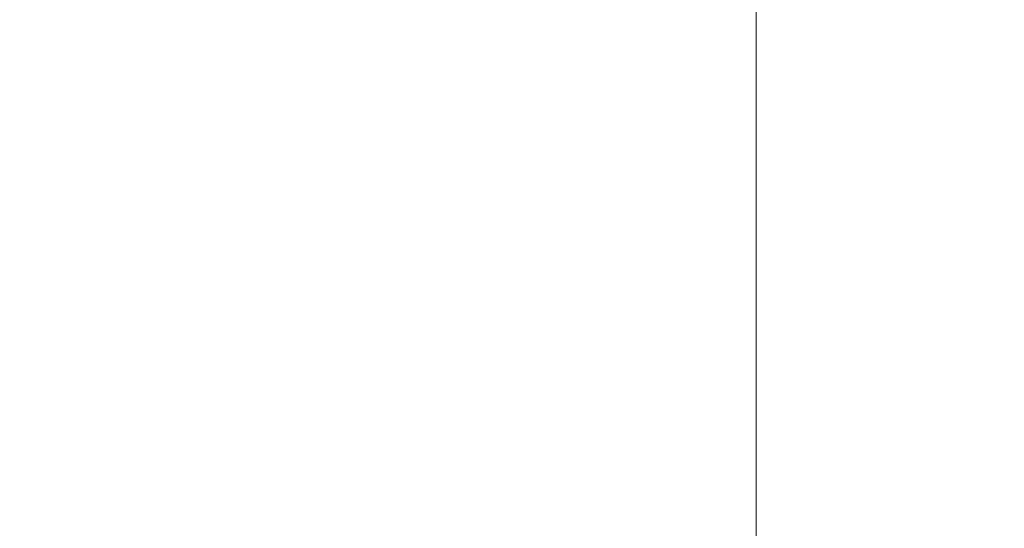
# Model space of a CAD drawing. Units: inches. Extents: x -466983 to 1020, y 324 to 318697.
# Tile 53 of 97: x 631.804 to 637.858, y 936.436 to 939.565. Entities that reach past the tile are written whole.
import ezdxf

# ---------------------------------------------------------------- set-up
doc = ezdxf.new("R2010")
doc.units = ezdxf.units.IN
doc.header["$MEASUREMENT"] = 0
doc.layers.add('A-FLOR-PATT', color=252, linetype='Continuous', lineweight=13)
doc.layers.add('A-FURN', color=8, linetype='Continuous', lineweight=18)

# ---------------------------------------------------------------- blocks, each defined once
blk = doc.blocks.new('L Shaped Sofa')
at = {"ltscale": 2}
blk.add_line((2432.347, 748.121), (2432.347, 765.179), dxfattribs=at)

msp = doc.modelspace()

# ---------------------------------------------------------------- hatches: boundary and pattern name
at = {"layer": 'A-FLOR-PATT', "transparency": 33554572}
h = msp.add_hatch(dxfattribs=at)
h.set_pattern_fill('ANSI37', color=256, scale=30)
h.set_pattern_definition([(45, (-1212.4137, -290.035), (-2.6516504, 2.6516504), []), (135, (-1212.4137, -290.035), (-2.6516504, -2.6516504), [])])
h.paths.add_polyline_path([(901.8057, 1075.9377), (900.6144, 1075.9377), (900.6144, 1065.3856), (899.391, 1065.3856), (898.0911, 1065.3856), (892.8356, 1058.7098, -0.258377), (892.1875, 1058.3509), (879.9848, 1058.3509, -0.20177), (879.4382, 1058.5808), (874.0812, 1065.3856), (872.7813, 1065.3856), (871.5579, 1065.3856), (871.5579, 1075.9377), (813.8057, 1075.9377), (813.8057, 1044.7922), (832.3947, 1044.7922, -0.394795), (848.6602, 1028.5356), (848.6602, 1009.9377), (901.8057, 1009.9377), (901.8057, 1015.9377), (901.3057, 1015.9377), (871.3057, 1015.9377), (871.3057, 1017.2502), (871.3344, 1017.2502, -0.401453), (901.3057, 1045.9377), (901.8057, 1045.9377)])
edge = h.paths.add_edge_path(flags=16)
edge.add_line((847.7731, 1068.9486), (847.7731, 1073.7088))
edge.add_arc((849.2269, 1073.7088), 1.4538, 90, 180, ccw=False)
edge.add_line((849.2269, 1075.1627), (864.4921, 1075.1627))
edge.add_arc((864.4921, 1073.7088), 1.4538, 0, 90, ccw=False)
edge.add_line((865.9459, 1073.7088), (865.9459, 1069.0035))
edge.add_arc((832.6447, 1068.9761), 33.3012, -20.61234, 0.04725, ccw=False)
edge.add_ellipse((856.8595, 1058.48), major_axis=(0, 10.2131), ratio=0.6859192, start_angle=100.00884, end_angle=259.99116, ccw=False)
edge.add_arc((881.0742, 1068.9761), 33.3012, 180.04725, 200.61234, ccw=False)
h.paths.add_polyline_path([(853.1456, 1066.4815), (853.1456, 1066.4534), (853.1463, 1066.4534, 0.433107), (852.9166, 1066.6849), (852.9166, 1066.4534), (853.1456, 1066.4534), (853.1456, 1066.4815), (853.088, 1066.6122, 0.697939), (852.6995, 1066.4534), (852.7003, 1066.4534), (852.7003, 1066.4815), (852.9166, 1067.0012), (852.9166, 1066.6849, -0.396254)], flags=0)
h.paths.add_polyline_path([(861.0187, 1066.4815), (861.0187, 1066.4534), (861.0194, 1066.4534, 0.416404), (860.8024, 1066.6849), (860.8024, 1066.4534), (861.0187, 1066.4534), (861.0187, 1066.4815), (860.9672, 1066.6053, 0.713344), (860.5726, 1066.4534), (860.5734, 1066.4534), (860.5734, 1066.4815), (860.8024, 1067.0012), (860.8024, 1066.6849, -0.379973)], flags=0)
edge = h.paths.add_edge_path(flags=0)
edge.add_spline(control_points=[(861.1298, 1065.7855), (861.4661, 1065.2478), (861.6134, 1065.0161), (861.9833, 1064.3736), (862.1924, 1063.9443), (862.5614, 1063.0391), (862.7212, 1062.5633), (862.9865, 1061.5781), (863.092, 1061.0689), (863.2452, 1060.031), (863.293, 1059.5025), (863.3295, 1058.4409), (863.3181, 1057.9078), (863.2366, 1056.8518), (863.1664, 1056.3289), (862.9695, 1055.308), (862.8427, 1054.8099), (862.5365, 1053.8522), (862.3571, 1053.3927), (861.9514, 1052.5249), (861.7251, 1052.1166), (861.233, 1051.3622), (860.9672, 1051.0162), (860.4048, 1050.3949), (860.1082, 1050.1197), (859.4937, 1049.6461), (859.1758, 1049.4476), (858.5276, 1049.1299), (858.1973, 1049.0107), (857.5315, 1048.8518), (857.1959, 1048.8121), (856.5249, 1048.812), (856.1894, 1048.8515), (855.5236, 1049.0101), (855.1933, 1049.1291), (854.545, 1049.4465), (854.2271, 1049.6449), (853.6124, 1050.1183), (853.3158, 1050.3933), (852.7533, 1051.0143), (852.4874, 1051.3602), (851.9952, 1052.1144), (851.7688, 1052.5225), (851.3629, 1053.3902), (851.1834, 1053.8496), (850.877, 1054.8071), (850.7501, 1055.3051), (850.553, 1056.326), (850.4827, 1056.8488), (850.401, 1057.9048), (850.3895, 1058.4379), (850.4257, 1059.4995), (850.4734, 1060.0281), (850.6265, 1061.066), (850.7318, 1061.5753), (850.9969, 1062.5605), (851.1567, 1063.0365), (851.5254, 1063.9418), (851.7345, 1064.3712), (852.1056, 1065.0164), (852.2544, 1065.2503), (852.6082, 1065.7335)], knot_values=[3.915332, 3.915332, 3.915332, 3.915332, 4.013468, 4.013468, 4.175532, 4.175532, 4.337596, 4.337596, 4.49966, 4.49966, 4.661724, 4.661724, 4.823788, 4.823788, 4.985852, 4.985852, 5.147916, 5.147916, 5.30998, 5.30998, 5.472044, 5.472044, 5.634109, 5.634109, 5.796173, 5.796173, 5.958237, 5.958237, 6.120301, 6.120301, 6.282365, 6.282365, 6.444429, 6.444429, 6.606493, 6.606493, 6.768557, 6.768557, 6.930621, 6.930621, 7.092685, 7.092685, 7.254749, 7.254749, 7.416813, 7.416813, 7.578878, 7.578878, 7.740942, 7.740942, 7.903006, 7.903006, 8.06507, 8.06507, 8.227134, 8.227134, 8.389198, 8.389198, 8.551262, 8.551262, 8.65037, 8.65037, 8.65037, 8.65037], degree=3, periodic=0)
edge.add_line((852.6421, 1065.7855), (861.1298, 1065.7855))
edge = h.paths.add_edge_path(flags=0)
edge.add_ellipse((856.8496, 1057.7432), major_axis=(0, 7.7921), ratio=0.687861, start_angle=0, end_angle=360)
h.paths.add_polyline_path([(848.8634, 1069.3891), (848.8634, 1073.9605, -0.414214), (849.9538, 1075.0508), (863.7652, 1075.0508, -0.414214), (864.8555, 1073.9605), (864.8555, 1069.3891, -0.388936), (864.5237, 1069.027, -0.043561), (849.1953, 1069.027, -0.388936)], flags=0)
h.paths.add_polyline_path([(853.1006, 1068.1122, -1), (852.6775, 1068.1122, -1)], flags=0)
edge = h.paths.add_edge_path(flags=0)
edge.add_ellipse((856.8595, 1057.3378), major_axis=(0, 2.207), ratio=0.657164, start_angle=0, end_angle=360)
h.paths.add_polyline_path([(861.0415, 1068.1122, -1), (860.6184, 1068.1122, -1)], flags=0)
edge = h.paths.add_edge_path()
edge.add_line((573.9537, 1057.3412), (573.9537, 1075.9377))
edge.add_line((573.9537, 1075.9377), (558.7308, 1075.9377))
edge.add_line((558.7308, 1075.9377), (558.7308, 1065.3856))
edge.add_line((558.7308, 1065.3856), (557.5074, 1065.3856))
edge.add_line((557.5074, 1065.3856), (556.2075, 1065.3856))
edge.add_line((556.2075, 1065.3856), (550.952, 1058.7098))
edge.add_arc((550.3039, 1059.1155), 0.7646, 270, 327.94832, ccw=False)
edge.add_line((550.3039, 1058.3509), (538.1012, 1058.3509))
edge.add_arc((538.1012, 1059.1155), 0.7646, 224.3704, 270, ccw=False)
edge.add_line((537.5546, 1058.5808), (532.1976, 1065.3856))
edge.add_line((532.1976, 1065.3856), (530.8977, 1065.3856))
edge.add_line((530.8977, 1065.3856), (529.6743, 1065.3856))
edge.add_line((529.6743, 1065.3856), (529.6743, 1075.9377))
edge.add_line((529.6743, 1075.9377), (520.8057, 1075.9377))
edge.add_line((520.8057, 1075.9377), (520.8057, 1045.9377))
edge.add_line((520.8057, 1045.9377), (521.3057, 1045.9377))
edge.add_arc((521.3057, 1015.9377), 30, 2.50749, 90, ccw=False)
edge.add_line((551.277, 1017.2502), (551.3057, 1017.2502))
edge.add_line((551.3057, 1017.2502), (551.3057, 1015.9377))
edge.add_line((551.3057, 1015.9377), (520.8057, 1015.9377))
edge.add_line((520.8057, 1015.9377), (520.8057, 1009.9377))
edge.add_line((520.8057, 1009.9377), (559.1913, 1010.4022))
edge.add_arc((559.1913, 1011.856), 1.4538, 180, 270, ccw=False)
edge.add_line((557.7375, 1011.856), (557.7375, 1016.5613))
edge.add_arc((591.0386, 1016.5888), 33.3012, 159.38766, 180.04725, ccw=False)
edge.add_ellipse((566.8239, 1027.0848), major_axis=(0, 10.2131), ratio=0.6859192, start_angle=280.00884, end_angle=439.99116, ccw=False)
edge.add_arc((542.6091, 1016.5888), 33.3012, 0.04725, 20.61234, ccw=False)
edge.add_line((575.9103, 1016.6162), (575.9103, 1011.856))
edge.add_arc((574.4565, 1011.856), 1.4538, -90, 0, ccw=False)
edge.add_line((574.4565, 1010.4022), (608.8057, 1009.9377))
edge.add_line((608.8057, 1009.9377), (608.8057, 1041.0857))
edge.add_line((608.8057, 1041.0857), (590.2179, 1041.0857))
edge.add_arc((590.775, 1057.9074), 16.8309, 181.92775, 268.10321, ccw=False)
edge = h.paths.add_edge_path()
edge.add_ellipse((494.2443, 583.6204), major_axis=(0, 10.2131), ratio=0.6859192, start_angle=280.00884, end_angle=439.99116, ccw=False)
edge.add_arc((470.0296, 573.1243), 33.3012, 0.04725, 20.61234, ccw=False)
edge.add_line((503.3307, 573.1518), (503.3307, 568.3916))
edge.add_arc((501.8769, 568.3916), 1.4538, -90, 0, ccw=False)
edge.add_line((501.8769, 566.9377), (539.8057, 566.9377))
edge.add_line((539.8057, 566.9377), (539.8057, 572.9377))
edge.add_line((539.8057, 572.9377), (539.3057, 572.9377))
edge.add_line((539.3057, 572.9377), (509.3057, 572.9377))
edge.add_line((509.3057, 572.9377), (509.3057, 574.2502))
edge.add_line((509.3057, 574.2502), (509.3344, 574.2502))
edge.add_arc((539.3057, 572.9377), 30, 90, 177.49251, ccw=False)
edge.add_line((539.3057, 602.9377), (539.8057, 602.9377))
edge.add_line((539.8057, 602.9377), (539.8057, 626.9377))
edge.add_line((539.8057, 626.9377), (531.7718, 626.9377))
edge.add_line((531.7718, 626.9377), (531.7718, 616.3856))
edge.add_line((531.7718, 616.3856), (530.5484, 616.3856))
edge.add_line((530.5484, 616.3856), (529.2485, 616.3856))
edge.add_line((529.2485, 616.3856), (523.7105, 609.3509))
edge.add_line((523.7105, 609.3509), (510.7766, 609.3509))
edge.add_line((510.7766, 609.3509), (505.2386, 616.3856))
edge.add_line((505.2386, 616.3856), (503.9387, 616.3856))
edge.add_line((503.9387, 616.3856), (502.7153, 616.3856))
edge.add_line((502.7153, 616.3856), (502.7153, 626.9377))
edge.add_line((502.7153, 626.9377), (481.6983, 626.9377))
edge.add_line((481.6983, 626.9377), (481.6983, 610.995))
edge.add_arc((467.2703, 611.4728), 14.4359, 271.92775, 358.10321, ccw=False)
edge.add_line((467.7559, 597.0451), (451.8057, 597.0451))
edge.add_line((451.8057, 597.0451), (451.8057, 584.4035))
edge.add_line((451.8057, 584.4035), (451.8057, 566.9377))
edge.add_line((451.8057, 566.9377), (486.6117, 566.9377))
edge.add_arc((486.6117, 568.3916), 1.4538, 180, 270, ccw=False)
edge.add_line((485.1579, 568.3916), (485.1579, 573.0969))
edge.add_arc((518.4591, 573.1243), 33.3012, 159.38766, 180.04725, ccw=False)
h.paths.add_polyline_path([(836.2609, 1020.7328), (879.8898, 1020.7328), (879.8898, 1039.3902), (836.2609, 1039.3902)], flags=25)
h.paths.add_polyline_path([(549.9851, 1036.7492), (593.614, 1036.7492), (593.614, 1055.4065), (549.9851, 1055.4065)], flags=24)
h.paths.add_polyline_path([(475.123, 595.5959), (518.752, 595.5959), (518.752, 614.2532), (475.123, 614.2532)], flags=24)
h = msp.add_hatch(dxfattribs=at)
h.set_pattern_fill('ANSI37', color=256, scale=20)
h.set_pattern_definition([(45, (-1212.4137, -290.035), (-1.767767, 1.767767), []), (135, (-1212.4137, -290.035), (-1.767767, -1.767767), [])])
h.paths.add_polyline_path([(809.8057, 870.9377), (809.8057, 888.1519), (806.9985, 888.1519), (802.6624, 888.1519), (789.3832, 888.1519), (786.2846, 888.1519, -0.414214), (785.4991, 888.9374), (785.4991, 900.1959), (785.4991, 908.4696, -0.414214), (786.8082, 909.7787, -0.414214), (785.4991, 911.0878), (785.4991, 929.1015, -0.414214), (786.8082, 930.4106, -0.414214), (785.4991, 931.7197), (785.4991, 931.9039, -0.414214), (784.19, 930.5948), (766.7223, 930.5948, -0.412359), (765.4132, 931.8956, -0.413741), (764.1145, 930.5782), (744.5781, 930.422, -0.416556), (743.7864, 931.2075), (743.7864, 933.5153), (742.2154, 933.5153), (742.2154, 952.024, -0.001344), (743.7864, 952.1998), (743.7864, 953.9377), (678.5915, 953.9377), (678.5915, 951.1305), (678.5915, 946.7945), (678.5915, 933.5153), (678.5915, 930.4166, -0.414214), (677.806, 929.6312), (666.5475, 929.6312), (658.2738, 929.6312, -0.414214), (656.9647, 930.9403, -0.414214), (655.6556, 929.6312), (637.6419, 929.6312, -0.414214), (636.3328, 930.9403, -0.414214), (635.0237, 929.6312), (634.8395, 929.6312, -0.414214), (636.1486, 928.322), (636.1486, 910.8544, -0.412359), (634.8478, 909.5452, -0.413741), (636.1653, 908.2466), (636.3214, 888.7102, -0.416556), (635.5359, 887.9184), (633.2281, 887.9184), (633.2281, 886.3475), (614.7194, 886.3475, -0.001344), (614.5436, 887.9184), (612.8057, 887.9184), (612.8057, 834.9377), (612.8057, 752.9377), (612.8057, 748.9377), (612.8057, 697.9377), (654.8057, 697.9377), (654.8057, 701.9377), (715.8057, 701.9377), (715.8057, 737.4353), (774.2918, 737.4353), (774.2918, 795.9377), (809.8057, 795.9377)])
h.paths.add_polyline_path([(679.2761, 849.5757, 0.102523), (682.1475, 849.2608, -0.080461), (694.5428, 849.7725, -0.283899), (694.4822, 849.0082, 0.136605), (694.4068, 848.8103, -0.030441), (694.5428, 846.8929), (694.5428, 842.6198), (694.5428, 838.3466, -0.028219), (694.4246, 836.5684), (694.425, 836.5684, 0.196187), (694.4456, 836.2708, -0.302897), (694.5428, 835.467, -0.080461), (682.1475, 835.9787, 0.102523), (679.2761, 835.6638, -0.58611), (678.6457, 836.0169), (678.6457, 849.2227, -0.58611)], flags=16)
h.paths.add_polyline_path([(679.5173, 848.6515, 0.699597), (679.476, 848.6342, 1.20716), (679.1935, 848.7422, 0.010621)], flags=0)
h.paths.add_polyline_path([(679.4923, 836.5608, -0.013798), (679.9178, 836.6594, -0.071703), (682.8533, 837.1434, -0.165743), (682.1665, 839.1006), (682.1665, 842.6094), (682.1665, 846.0603, -0.240616), (683.4733, 848.6767, -0.068263), (693.9295, 849.0082), (693.7875, 848.7083), (693.7875, 849.0228, 0.067332), (683.4733, 848.6767, 0.240616), (682.1665, 846.0603), (682.1665, 842.6094), (682.1665, 839.1006, 0.23459), (683.461, 836.5513, 0.068093), (693.7875, 836.1955), (693.7875, 836.5104), (693.9296, 836.2102, -0.077215), (682.2421, 836.7815, 0.086627), (679.5283, 836.5701, -0.628402), (679.5029, 836.5735), (679.5029, 836.6071, 0.910458)], flags=0)
h.paths.add_polyline_path([(679.476, 848.6364), (679.2069, 848.647), (679.2069, 836.5718, 0.913566), (679.3645, 836.5861), (679.476, 836.5824)], flags=0)
h.paths.add_polyline_path([(679.2761, 829.8604, 0.102523), (682.1475, 829.5455, -0.080461), (694.5428, 830.0572, -0.283899), (694.4822, 829.2929, 0.136605), (694.4068, 829.095, -0.030441), (694.5428, 827.1776), (694.5428, 822.9045), (694.5428, 818.6314, -0.028219), (694.4246, 816.8531), (694.425, 816.8532, 0.196187), (694.4456, 816.5555, -0.302897), (694.5428, 815.7517, -0.080461), (682.1475, 816.2635, 0.102523), (679.2761, 815.9485, -0.58611), (678.6457, 816.3016), (678.6457, 829.5074, -0.58611)], flags=16)
h.paths.add_polyline_path([(679.5173, 828.9362, 0.699597), (679.476, 828.9189, 1.20716), (679.1935, 829.0269, 0.010621)], flags=0)
h.paths.add_polyline_path([(679.4923, 816.8456, -0.013798), (679.9178, 816.9441, -0.071703), (682.8533, 817.4281, -0.165743), (682.1665, 819.3853), (682.1665, 822.8941), (682.1665, 826.345, -0.240616), (683.4733, 828.9614, -0.068263), (693.9295, 829.2929), (693.7875, 828.9931), (693.7875, 829.3076, 0.067332), (683.4733, 828.9614, 0.240616), (682.1665, 826.345), (682.1665, 822.8941), (682.1665, 819.3853, 0.23459), (683.461, 816.836, 0.068093), (693.7875, 816.4802), (693.7875, 816.7952), (693.9296, 816.4949, -0.077215), (682.2421, 817.0662, 0.086627), (679.5283, 816.8549, -0.628402), (679.5029, 816.8582), (679.5029, 816.8918, 0.910458)], flags=0)
h.paths.add_polyline_path([(679.476, 828.9211), (679.2069, 828.9317), (679.2069, 816.8565, 0.913566), (679.3645, 816.8708), (679.476, 816.8671)], flags=0)
h.paths.add_polyline_path([(679.2761, 810.1451, 0.102523), (682.1475, 809.8302, -0.080461), (694.5428, 810.342, -0.3023), (694.4466, 809.5394, 0.10023), (694.4058, 809.3878, -0.03057), (694.5428, 807.4623), (694.5428, 803.1892), (694.5428, 798.9161, -0.03057), (694.4058, 796.9906, 0.10023), (694.4466, 796.839, -0.3023), (694.5428, 796.0365, -0.080461), (682.1475, 796.5482, 0.102523), (679.2761, 796.2333, -0.58611), (678.6457, 796.5863), (678.6457, 809.7921, -0.58611)], flags=16)
h.paths.add_polyline_path([(679.5173, 809.2417, 0.699597), (679.476, 809.2244, 1.20716), (679.1935, 809.3324, 0.010621)], flags=0)
h.paths.add_polyline_path([(679.4923, 797.151, -0.013798), (679.9178, 797.2496, -0.071703), (682.8533, 797.7336, -0.165743), (682.1665, 799.6908), (682.1665, 803.1996), (682.1665, 806.6505, -0.239349), (683.461, 809.2577, -0.072465), (694.4468, 809.5405, 0.197932), (694.425, 809.2405), (693.7875, 809.2985), (693.7875, 809.6135, 0.068093), (683.461, 809.2577, 0.239349), (682.1665, 806.6505), (682.1665, 803.1996), (682.1665, 799.6908, 0.235854), (683.4733, 797.1323, 0.067332), (693.7875, 796.7861), (693.7875, 797.1006), (694.425, 797.1586, 0.197932), (694.4468, 796.8586, -0.080419), (682.1557, 797.3795, 0.083867), (679.5283, 797.1603, -0.628402), (679.5029, 797.1637), (679.5029, 797.1973, 0.910458)], flags=0)
h.paths.add_polyline_path([(679.2069, 809.2372), (679.2069, 797.162, 0.913566), (679.3645, 797.1763), (679.476, 797.1726), (679.476, 809.2266)], flags=0)
h.paths.add_polyline_path([(695.3643, 853.2989), (728.2231, 853.2989), (728.2231, 771.1519), (695.3643, 771.1519)], flags=16)
h.paths.add_polyline_path([(696.0215, 852.6417), (727.5659, 852.6417), (727.5659, 771.809), (696.0215, 771.809)], flags=0)
h.paths.add_polyline_path([(679.2761, 788.7869, 0.102523), (682.1475, 788.472, -0.080461), (694.5428, 788.9837, -0.3023), (694.4466, 788.1812, 0.10023), (694.4058, 788.0296, -0.03057), (694.5428, 786.1041), (694.5428, 781.831), (694.5428, 777.5578, -0.03057), (694.4058, 775.6323, 0.10023), (694.4466, 775.4808, -0.3023), (694.5428, 774.6782, -0.080461), (682.1475, 775.19, 0.102523), (679.2761, 774.875, -0.58611), (678.6457, 775.2281), (678.6457, 788.4339, -0.58611)], flags=16)
h.paths.add_polyline_path([(679.5173, 787.8834, 0.699597), (679.476, 787.8662, 1.20716), (679.1935, 787.9742, 0.010621)], flags=0)
h.paths.add_polyline_path([(679.4923, 775.7928, -0.013798), (679.9178, 775.8914, -0.071703), (682.8533, 776.3753, -0.165743), (682.1665, 778.3325), (682.1665, 781.8414), (682.1665, 785.2922, -0.239349), (683.461, 787.8995, -0.072465), (694.4468, 788.1823, 0.197932), (694.425, 787.8823), (693.7875, 787.9403), (693.7875, 788.2553, 0.068093), (683.461, 787.8995, 0.239349), (682.1665, 785.2922), (682.1665, 781.8414), (682.1665, 778.3325, 0.235854), (683.4733, 775.7741, 0.067332), (693.7875, 775.4279), (693.7875, 775.7424), (694.425, 775.8004, 0.197932), (694.4468, 775.5004, -0.080419), (682.1557, 776.0212, 0.083867), (679.5283, 775.8021, -0.628402), (679.5029, 775.8054), (679.5029, 775.8391, 0.910458)], flags=0)
h.paths.add_polyline_path([(679.2069, 787.8789), (679.2069, 775.8038, 0.913566), (679.3645, 775.818), (679.476, 775.8144), (679.476, 787.8684)], flags=0)
h.paths.add_polyline_path([(704.641, 854.1204, -0.080461), (705.1527, 866.5157, 0.102523), (704.8378, 869.3871, -0.58611), (705.1908, 870.0174), (718.3966, 870.0174, -0.58611), (718.7496, 869.3871, 0.102523), (718.4347, 866.5157, -0.080461), (718.9465, 854.1204, -0.3023), (718.1439, 854.2166, 0.10023), (717.9924, 854.2574, -0.03057), (716.0668, 854.1204), (711.7937, 854.1204), (707.5206, 854.1204, -0.03057), (705.5951, 854.2574, 0.10023), (705.4435, 854.2166, -0.3023)], flags=16)
h.paths.add_polyline_path([(717.8462, 869.1459, 0.699597), (717.8289, 869.1872, 1.20716), (717.9369, 869.4697, 0.010621)], flags=0)
h.paths.add_polyline_path([(705.4631, 854.2164, -0.080419), (705.984, 866.5074, 0.083867), (705.7648, 869.1349, -0.628402), (705.7682, 869.1603), (705.8018, 869.1603, 0.910458), (705.7555, 869.1709, -0.013798), (705.8541, 868.7454, -0.071703), (706.3381, 865.8099, -0.165743), (708.2953, 866.4967), (711.8041, 866.4967), (715.255, 866.4967, -0.239349), (717.8622, 865.2022, -0.072465), (718.145, 854.2164, 0.197932), (717.845, 854.2382), (717.903, 854.8757), (718.218, 854.8757, 0.068093), (717.8622, 865.2022, 0.239349), (715.255, 866.4967), (711.8041, 866.4967), (708.2953, 866.4967, 0.235854), (705.7368, 865.1898, 0.067332), (705.3906, 854.8757), (705.7051, 854.8757), (705.7631, 854.2382, 0.197932)], flags=16)
h.paths.add_polyline_path([(705.7665, 869.4563, 0.913566), (705.7808, 869.2987), (705.7771, 869.1872), (717.8311, 869.1872), (717.8417, 869.4563)], flags=0)
h.paths.add_polyline_path([(729.0446, 842.6198), (729.0446, 846.8929, -0.03057), (729.1817, 848.8184, 0.10023), (729.1408, 848.9699, -0.3023), (729.0446, 849.7725, -0.080461), (741.4399, 849.2608, 0.102523), (744.3113, 849.5757, -0.58611), (744.9417, 849.2227), (744.9417, 836.0169, -0.58611), (744.3113, 835.6638, 0.102523), (741.4399, 835.9787, -0.080461), (729.0446, 835.467, -0.3023), (729.1408, 836.2696, 0.10023), (729.1817, 836.4211, -0.03057), (729.0446, 838.3466)], flags=16)
h.paths.add_polyline_path([(744.1115, 836.5846, 1.20716), (744.3939, 836.4766, 0.010621), (744.0701, 836.5673, 0.699597)], flags=0)
h.paths.add_polyline_path([(729.1407, 836.2684, 0.197932), (729.1624, 836.5684), (729.7999, 836.5104), (729.7999, 836.1955, 0.068093), (740.1264, 836.5513, 0.239349), (741.4209, 839.1585), (741.4209, 842.6094), (741.4209, 846.1182, 0.235854), (740.1141, 848.6767, 0.067332), (729.7999, 849.0228), (729.7999, 848.7083), (729.1624, 848.6503, 0.197932), (729.1407, 848.9504, -0.080419), (741.4317, 848.4295, 0.083867), (744.0591, 848.6486, -0.628402), (744.0845, 848.6453), (744.0845, 848.6117, 0.910458), (744.0951, 848.6579, -0.013798), (743.6696, 848.5594, -0.071703), (740.7341, 848.0754, -0.165743), (741.4209, 846.1182), (741.4209, 842.6094), (741.4209, 839.1585, -0.239349), (740.1264, 836.5513, -0.072465)], flags=0)
h.paths.add_polyline_path([(729.0446, 830.0572, -0.080461), (741.4399, 829.5455, 0.102523), (744.3113, 829.8604, -0.58611), (744.9417, 829.5074), (744.9417, 816.3016, -0.58611), (744.3113, 815.9485, 0.102523), (741.4399, 816.2635, -0.080461), (729.0446, 815.7517, -0.3023), (729.1408, 816.5543, 0.10023), (729.1817, 816.7058, -0.03057), (729.0446, 818.6314), (729.0446, 822.9045), (729.0446, 827.1776, -0.03057), (729.1817, 829.1031, 0.10023), (729.1408, 829.2547, -0.3023)], flags=16)
h.paths.add_polyline_path([(744.1115, 816.8693, 1.20716), (744.3939, 816.7613, 0.010621), (744.0701, 816.852, 0.699597)], flags=0)
h.paths.add_polyline_path([(729.1407, 829.2351, -0.080419), (741.4317, 828.7142, 0.083867), (744.0591, 828.9334, -0.628402), (744.0845, 828.93), (744.0845, 828.8964, 0.910458), (744.0951, 828.9427, -0.013798), (743.6696, 828.8441, -0.071703), (740.7341, 828.3601, -0.165743), (741.4209, 826.4029), (741.4209, 822.8941), (741.4209, 819.4432, -0.239349), (740.1264, 816.836, -0.072465), (729.1407, 816.5531, 0.197932), (729.1624, 816.8532), (729.7999, 816.7952), (729.7999, 816.4802, 0.068093), (740.1264, 816.836, 0.239349), (741.4209, 819.4432), (741.4209, 822.8941), (741.4209, 826.4029, 0.235854), (740.1141, 828.9614, 0.067332), (729.7999, 829.3076), (729.7999, 828.9931), (729.1624, 828.9351, 0.197932)], flags=16)
h.paths.add_polyline_path([(729.0446, 810.342, -0.080461), (741.4399, 809.8302, 0.102523), (744.3113, 810.1451, -0.58611), (744.9417, 809.7921), (744.9417, 796.5863, -0.58611), (744.3113, 796.2333, 0.102523), (741.4399, 796.5482, -0.080461), (729.0446, 796.0365, -0.283899), (729.1052, 796.8007, 0.136605), (729.1806, 796.9987, -0.030441), (729.0446, 798.9161), (729.0446, 803.1892), (729.0446, 807.4623, -0.028219), (729.1628, 809.2406), (729.1624, 809.2405, 0.196187), (729.1418, 809.5382, -0.302897)], flags=16)
h.paths.add_polyline_path([(744.1115, 797.1748, 1.20716), (744.3939, 797.0668, 0.010621), (744.0701, 797.1575, 0.699597)], flags=0)
h.paths.add_polyline_path([(741.3453, 809.0275, 0.086627), (744.0591, 809.2388, -0.628402), (744.0845, 809.2355), (744.0845, 809.2019, 0.910458), (744.0951, 809.2481, -0.013798), (743.6696, 809.1496, -0.071703), (740.7341, 808.6656, -0.165743), (741.4209, 806.7084), (741.4209, 803.1996), (741.4209, 799.7487, -0.240616), (740.1141, 797.1323, -0.068263), (729.658, 796.8008), (729.7999, 797.1006), (729.7999, 796.7861, 0.067332), (740.1141, 797.1323, 0.240616), (741.4209, 799.7487), (741.4209, 803.1996), (741.4209, 806.7084, 0.23459), (740.1264, 809.2577, 0.068093), (729.7999, 809.6135), (729.7999, 809.2985), (729.6578, 809.5988, -0.077215)], flags=0)
h.paths.add_polyline_path([(704.641, 770.3304, -0.283899), (705.4053, 770.2697, 0.136605), (705.6032, 770.1944, -0.030441), (707.5206, 770.3304), (711.7937, 770.3304), (716.0668, 770.3304, -0.028219), (717.8451, 770.2122), (717.845, 770.2126, 0.196187), (718.1427, 770.2331, -0.302897), (718.9465, 770.3304, -0.080461), (718.4347, 757.9351, 0.102523), (718.7496, 755.0637, -0.58611), (718.3966, 754.4333), (705.1908, 754.4333, -0.58611), (704.8378, 755.0637, 0.102523), (705.1527, 757.9351, -0.080461)], flags=16)
h.paths.add_polyline_path([(705.762, 755.3048, 0.699597), (705.7793, 755.2635, 1.20716), (705.6713, 754.9811, 0.010621)], flags=0)
h.paths.add_polyline_path([(705.4053, 769.717), (705.7051, 769.5751), (705.3906, 769.5751, 0.067332), (705.7368, 759.2609, 0.240616), (708.3532, 757.954), (711.8041, 757.954), (715.3129, 757.954, 0.23459), (717.8622, 759.2485, 0.068093), (718.218, 769.5751), (717.903, 769.5751), (718.2033, 769.7172, -0.077215), (717.632, 758.0297, 0.086627), (717.8433, 755.3159, -0.628402), (717.84, 755.2904), (717.8064, 755.2904, 0.910458), (717.8526, 755.2799, -0.013798), (717.7541, 755.7053, -0.071703), (717.2701, 758.6409, -0.165743), (715.3129, 757.954), (711.8041, 757.954), (708.3532, 757.954, -0.240616), (705.7368, 759.2609, -0.068263)], flags=0)
h.paths.add_polyline_path([(729.0446, 788.9837, -0.080461), (741.4399, 788.472, 0.102523), (744.3113, 788.7869, -0.58611), (744.9417, 788.4339), (744.9417, 775.2281, -0.58611), (744.3113, 774.875, 0.102523), (741.4399, 775.19, -0.080461), (729.0446, 774.6782, -0.283899), (729.1052, 775.4425, 0.136605), (729.1806, 775.6405, -0.030441), (729.0446, 777.5578), (729.0446, 781.831), (729.0446, 786.1041, -0.028219), (729.1628, 787.8823), (729.1624, 787.8823, 0.196187), (729.1418, 788.1799, -0.302897)], flags=16)
h.paths.add_polyline_path([(744.1115, 775.8165, 1.20716), (744.3939, 775.7086, 0.010621), (744.0701, 775.7993, 0.699597)], flags=0)
h.paths.add_polyline_path([(741.3453, 787.6692, 0.086627), (744.0591, 787.8806, -0.628402), (744.0845, 787.8773), (744.0845, 787.8437, 0.910458), (744.0951, 787.8899, -0.013798), (743.6696, 787.7913, -0.071703), (740.7341, 787.3074, -0.165743), (741.4209, 785.3502), (741.4209, 781.8414), (741.4209, 778.3905, -0.240616), (740.1141, 775.7741, -0.068263), (729.658, 775.4425), (729.7999, 775.7424), (729.7999, 775.4279, 0.067332), (740.1141, 775.7741, 0.240616), (741.4209, 778.3905), (741.4209, 781.8414), (741.4209, 785.3502, 0.23459), (740.1264, 787.8995, 0.068093), (729.7999, 788.2553), (729.7999, 787.9403), (729.6578, 788.2405, -0.077215)], flags=0)
h.paths.add_polyline_path([(744.1115, 848.6364), (744.1115, 836.5824), (744.3805, 836.5718), (744.3805, 848.647, 0.913566), (744.2229, 848.6327)], flags=0)
h.paths.add_polyline_path([(744.2229, 828.9174), (744.1115, 828.9211), (744.1115, 816.8671), (744.3805, 816.8565), (744.3805, 828.9317, 0.913566)], flags=0)
h.paths.add_polyline_path([(717.8311, 755.2635), (705.7771, 755.2635), (705.7665, 754.9945), (717.8417, 754.9945, 0.913566), (717.8274, 755.1521)], flags=0)
h.paths.add_polyline_path([(744.2229, 809.2229), (744.1115, 809.2266), (744.1115, 797.1726), (744.3805, 797.162), (744.3805, 809.2372, 0.913566)], flags=0)
h.paths.add_polyline_path([(744.1115, 787.8684), (744.1115, 775.8144), (744.3805, 775.8038), (744.3805, 787.8789, 0.913566), (744.2229, 787.8647)], flags=0)
h.paths.add_polyline_path([(678.8774, 877.1228), (737.6127, 877.1228), (737.6127, 899.5116), (678.8774, 899.5116)], flags=24)

# ---------------------------------------------------------------- linework, layer by layer
at = {"layer": 'A-FURN', "ltscale": 2}
msp.add_line((636.3328, 940.2915), (636.3328, 930.9403), dxfattribs=at)
msp.add_line((636.3328, 940.2915), (636.3328, 930.9403), dxfattribs=at)
msp.add_line((636.3328, 940.2915), (636.3328, 930.9403), dxfattribs=at)
msp.add_line((636.3328, 940.2915), (636.3328, 930.9403), dxfattribs=at)
msp.add_line((636.3328, 940.2915), (636.3328, 930.9403), dxfattribs=at)
msp.add_line((636.3328, 940.2915), (636.3328, 930.9403), dxfattribs=at)

# ---------------------------------------------------------------- block references
at = {"layer": 'A-FURN', "xscale": 0.5482153745360612, "yscale": 0.5482153745360612, "zscale": 0.5482153745360612, "rotation": 180}
msp.add_blockref('L Shaped Sofa', (1969.7828, 1350.4232), dxfattribs=at)

doc.saveas('drawing.dxf')
